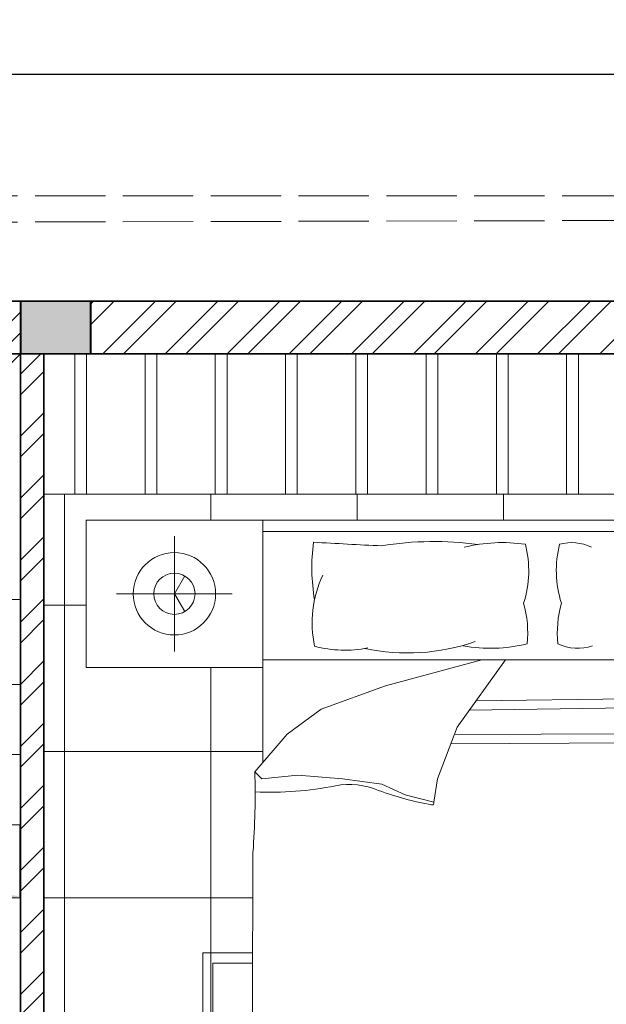
# Model space of a CAD drawing. Units: inches. Extents: x 351 to 1738, y -265 to 286.
# Tile 36 of 38: x 1380 to 1480, y 118 to 286. Entities that reach past the tile are written whole.
import ezdxf

# ---------------------------------------------------------------- set-up
doc = ezdxf.new("R2010")
doc.units = ezdxf.units.IN
doc.header["$MEASUREMENT"] = 0
doc.linetypes.add('ACAD_ISO02W100', pattern=[15, 12, -3])
for name, color, linetype, lineweight in [('A-ANNO-DIMS', 2, 'Continuous', 18), ('A-COLS', 7, 'Continuous', 40), ('A-COLS-PATT', 6, 'Continuous', 13), ('A-FLOR-CASE', 9, 'Continuous', 18), ('A-FLOR-OVHD', 1, 'ACAD_ISO02W100', 18), ('A-FLOR-PATT', 9, 'Continuous', 9), ('A-FLOR-STRS', 7, 'Continuous', 18), ('A-FURN', 18, 'Continuous', 13), ('A-WALL', 7, 'Continuous', 35), ('A-WALL-PATT', 152, 'Continuous', 13)]:
    doc.layers.add(name, color=color, linetype=linetype, lineweight=lineweight)
doc.styles.get("Standard").update_dxf_attribs({"font": 'arial.ttf'})
doc.dimstyles.get("Standard").update_dxf_attribs({"dimtxt": 8, "dimasz": 5, "dimexe": 0.18, "dimexo": 0.0625, "dimgap": 0.09, "dimtad": 1, "dimtoh": 1, "dimzin": 0, "dimdsep": 46, "dimlunit": 4, "dimtxsty": 'Standard', "dimcen": 0, "dimclre": 256, "dimadec": 0, "dimazin": 0, "dimtfac": 1, "dimtofl": 0, "dimtmove": 0, "dimatfit": 3, "dimfxl": 1, "dimtolj": 1, "dimtzin": 0, "dimlwe": -1, "dimarcsym": 0})

# ---------------------------------------------------------------- blocks, each defined once
blk = doc.blocks.new('*D7')
at = {"layer": 'A-ANNO-DIMS', "color": 0, "transparency": 16777216}
for p, q in [((1034.7, 256.03), (1034.7, 276.92)), ((1566.7, 256.03), (1566.7, 276.92))]:
    blk.add_line(p, q, dxfattribs=at)
at = {"layer": 'A-ANNO-DIMS', "color": 0, "lineweight": -2, "transparency": 16777216}
blk.add_line((1039.7, 276.74), (1561.7, 276.74), dxfattribs=at)
at = {"layer": 'A-ANNO-DIMS', "color": 0, "transparency": 16777216}
for points in [[(1039.7, 277.57), (1039.7, 275.91), (1034.7, 276.74)], [(1561.7, 277.57), (1561.7, 275.91), (1566.7, 276.74)]]:
    blk.add_solid(points, dxfattribs=at)
at = {"layer": 'Defpoints', "color": 0, "transparency": 16777216}
for p in [(1566.7, 276.74), (1034.7, 255.96), (1566.7, 255.96)]:
    blk.add_point(p, dxfattribs=at)
at = {"layer": 'A-ANNO-DIMS', "color": 0, "transparency": 16777216, "insert": (1300.7, 280.83), "char_height": 8, "attachment_point": 5}
blk.add_mtext('\\A1;44\'-4"', dxfattribs=at)
blk = doc.blocks.new('*D13')
at = {"layer": 'A-ANNO-DIMS', "color": 0, "transparency": 16777216}
for p, q in [((1338.06, 148.4), (1338.06, 136.03)), ((1380.06, 148.4), (1380.06, 136.03))]:
    blk.add_line(p, q, dxfattribs=at)
at = {"layer": 'A-ANNO-DIMS', "color": 0, "lineweight": -2, "transparency": 16777216}
blk.add_line((1343.06, 136.21), (1375.06, 136.21), dxfattribs=at)
at = {"layer": 'A-ANNO-DIMS', "color": 0, "transparency": 16777216}
for points in [[(1343.06, 137.05), (1343.06, 135.38), (1338.06, 136.21)], [(1375.06, 137.05), (1375.06, 135.38), (1380.06, 136.21)]]:
    blk.add_solid(points, dxfattribs=at)
at = {"layer": 'Defpoints', "color": 0, "transparency": 16777216}
for p in [(1338.06, 148.46), (1380.06, 148.46), (1380.06, 136.21)]:
    blk.add_point(p, dxfattribs=at)
at = {"layer": 'A-ANNO-DIMS', "color": 0, "transparency": 16777216, "insert": (1359.06, 140.39), "char_height": 8, "attachment_point": 5}
blk.add_mtext('\\A1;3\'-6"', dxfattribs=at)
blk = doc.blocks.new('BED-DOUBLE-W-NIGHTSTANDS')
for p, q in [((30.18, 128.33), (30.18, 86.91)), ((120.72, 126.39), (30.18, 126.39)), ((15.09, 105.9), (15.09, 125.61)), ((24.95, 115.76), (5.23, 115.76)), ((30.18, 104.48), (120.72, 104.48)), ((120.32, 98.22), (66.59, 97.46)), ((120.26, 96.67), (65.46, 95.89)), ((120.18, 91.92), (62.88, 91.69)), ((120.19, 90.37), (62.29, 90.13))]:
    blk.add_line(p, q)
for points in [[(30.18, 103.18), (0, 103.18), (0, 128.33), (150.9, 128.33), (150.9, 103.18), (120.72, 103.18), (120.72, 128.33)], [(16.85, 112.71), (15.09, 115.76), (16.85, 118.81)], [(71.64, 104.48), (63.37, 92.97), (60, 84.12), (59.39, 80.15), (54.5, 81.37), (50.53, 83.2), (43.81, 84.12), (36.16, 84.73), (30.05, 84.12), (28.83, 85.34), (34.33, 91.75), (40.14, 96.03), (51.14, 100), (67.6, 104.48)], [(121.56, 54.36), (129.93, 54.36), (129.93, 0), (19.92, 0), (19.92, 54.36), (28.45, 54.36)], [(28.45, 52.61), (21.67, 52.61), (21.67, 1.75), (128.18, 1.75), (128.18, 52.61), (121.53, 52.61)]]:
    blk.add_lwpolyline(points)
for points in [[(38.85, 124.57, 0.074897), (39.03, 114.71, -0.472817)], [(74.74, 114.16, 0.14099), (75.04, 124.22, 0.235245)], [(81.19, 114.16, -0.14099), (80.89, 124.22, -0.235245)], [(28.51, 71.52, 0.001242), (28.44, 42.89, -0.127202), (25.42, 28.62)]]:
    blk.add_lwpolyline(points, format="xyb")
for radius in [7.04, 3.52]:
    blk.add_circle((15.09, 115.76), radius)
for centre, radius, start, end in [((122.02, 1560.65), 1438.48, 266.68521, 267.14978), ((59.52, 69.97), 54.73, 82.2196, 99.497), ((71.08, 97.62), 26.89, 81.5249, 103.96), ((82.96, 117.05), 7.46, 63.3437, 106.1026), ((58.07, 110.76), 19.45, 155.1316, 191.7583), ((56.95, 109.12), 18.49, 354.0129, 15.8293), ((98.98, 109.12), 18.49, 164.1707, 185.9871), ((44.23, 126.34), 20.22, 255.1039, 281.0369), ((54.88, 140.71), 35.07, 258.0397, 289.2615), ((69.08, 133.05), 26.61, 259.8617, 283.6238), ((83.97, 114.44), 8, 245.0183, 288.5407), ((-109.53, 81.59), 138.41, 355.8294, 1.553), ((31.41, 138.78), 56.95, 267.4519, 281.3392), ((45.02, 70.89), 12.28, 66.2616, 101.3392), ((69.87, 137.17), 58.52, 250.1194, 259.3383), ((59.05, 80.02), 0.364, 268.8623, 19.7536)]:
    blk.add_arc(centre, radius, start, end)
blk = doc.blocks.new('WARDROBE-PANELLED')
for p, q in [((5.27, 24), (5.27, 0)), ((7.27, 24), (7.27, 0)), ((17.27, 24), (17.27, 0)), ((19.27, 24), (19.27, 0)), ((29.27, 24), (29.27, 0)), ((31.27, 24), (31.27, 0)), ((41.27, 24), (41.27, 0)), ((43.27, 24), (43.27, 0)), ((53.27, 24), (53.27, 0)), ((55.27, 24), (55.27, 0)), ((65.27, 24), (65.27, 0)), ((67.27, 24), (67.27, 0)), ((77.27, 24), (77.27, 0)), ((79.27, 24), (79.27, 0)), ((89.27, 24), (89.27, 0)), ((91.27, 24), (91.27, 0)), ((0, 0), (173.5, 0))]:
    blk.add_line(p, q)

msp = doc.modelspace()

# ---------------------------------------------------------------- hatches: boundary and pattern name
at = {"layer": 'A-COLS-PATT'}
h = msp.add_hatch(color=256, dxfattribs=at)
h.dxf.hatch_style = 1
h.paths.add_polyline_path([(1112.704, 237.963), (1103.704, 237.963), (1103.704, 228.963), (1112.704, 228.963)])
h.paths.add_polyline_path([(1115.704, 237.963), (1112.704, 237.963), (1112.704, 228.963), (1115.704, 228.963)])
h.paths.add_polyline_path([(1043.704, 255.963), (1034.704, 255.963), (1034.704, 243.963), (1043.704, 243.963)])
h.paths.add_polyline_path([(1043.704, 210.963), (1034.704, 210.963), (1034.704, 198.963), (1043.704, 198.963)])
h.paths.add_polyline_path([(1043.704, -45.037), (1034.704, -45.037), (1034.704, -57.037), (1043.704, -57.037)])
h.paths.add_polyline_path([(1112.704, -45.037), (1103.704, -45.037), (1103.704, -57.037), (1112.704, -57.037)])
h.paths.add_polyline_path([(1112.704, -161.037), (1103.704, -161.037), (1103.704, -164.037), (1103.704, -173.037), (1112.704, -173.037)])
h.paths.add_polyline_path([(1043.704, -161.037), (1034.704, -161.037), (1034.704, -173.037), (1043.704, -173.037)])
h.paths.add_polyline_path([(1248.549, -164.037), (1236.549, -164.037), (1236.549, -173.037), (1248.549, -173.037)])
h.paths.add_polyline_path([(1248.549, -50), (1236.549, -50), (1236.549, -59), (1248.549, -59)])
h.paths.add_polyline_path([(1248.704, 73.463), (1244.704, 73.463), (1244.704, 64.463), (1248.704, 64.463)])
h.paths.add_polyline_path([(1244.704, 73.463), (1236.704, 73.463), (1236.704, 64.463), (1244.704, 64.463)])
h.paths.add_polyline_path([(1248.704, 237.963), (1236.704, 237.963), (1236.704, 228.963), (1248.704, 228.963)])
h.paths.add_polyline_path([(1392.204, 237.963), (1380.204, 237.963), (1380.204, 228.963), (1392.204, 228.963)])
h.paths.add_polyline_path([(1536.064, 237.963), (1524.064, 237.963), (1524.064, 228.963), (1536.064, 228.963)])
h.paths.add_polyline_path([(1536.064, 73.463), (1524.064, 73.463), (1524.064, 64.463), (1536.064, 64.463)])
h.paths.add_polyline_path([(1384.204, 73.463), (1380.204, 73.463), (1380.204, 64.463), (1384.204, 64.463)])
h.paths.add_polyline_path([(1392.064, 73.463), (1384.204, 73.463), (1384.204, 64.463), (1392.064, 64.463)])
h.paths.add_polyline_path([(1536.064, -53.037), (1524.064, -53.037), (1524.064, -57.037), (1536.064, -57.037)])
h.paths.add_polyline_path([(1536.064, -48.037), (1524.064, -48.037), (1524.064, -53.037), (1536.064, -53.037)])
h.paths.add_polyline_path([(1392.064, -48.037), (1380.064, -48.037), (1380.064, -56.5), (1380.065, -57.037), (1392.064, -57.037)])
h.paths.add_polyline_path([(1536.064, -164.037), (1524.064, -164.037), (1524.064, -173.037), (1536.064, -173.037)])
at = {"layer": 'A-FLOR-PATT', "transparency": 33554559}
h = msp.add_hatch(dxfattribs=at)
h.set_pattern_fill('ANSI37', color=256, scale=200, angle=135)
h.set_pattern_definition([(180, (1112.704, -164.037), (-2e-15, -25), []), (270, (1112.704, -164.037), (25, -5e-15), [])])
h.paths.add_polyline_path([(1380.064, 73.463), (1380.132, 148.463), (1338.064, 148.463), (1290.704, 148.463), (1290.704, 88.463), (1248.704, 88.463), (1248.704, -2.009), (1244.704, -2.009), (1244.704, 142.457), (1160.704, 142.457), (1160.704, 158.963), (1160.704, 170.137), (1160.704, 206.137), (1160.704, 228.963), (1112.704, 228.963), (1112.704, 209.963), (1112.704, 168.963), (1124.704, 168.963), (1124.704, 162.963), (1112.704, 162.963), (1112.704, 64.463), (1112.704, 60.463), (1112.704, 0.463), (1112.704, -48.026), (1146.804, -47.981), (1146.804, -35.691), (1207.804, -35.691), (1207.804, -47.902), (1236.542, -47.864), (1236.544, -50.009), (1248.5, -50.009), (1248.506, -102.915), (1248.512, -150.915), (1248.514, -164.037), (1248.549, -164.037), (1273.017, -164.037), (1273.017, -128.799), (1355.24, -128.799), (1355.24, -164.037), (1384.204, -164.037), (1384.204, -57.037), (1380.064, -57.037), (1380.064, -48.037), (1392.064, -48.037), (1392.064, -53.037), (1406.549, -53.037), (1406.549, -57.037), (1401.204, -57.037), (1401.204, -147.037), (1468.204, -147.037), (1468.204, -138.5), (1472.204, -138.5), (1472.204, -102.5), (1468.204, -102.5), (1468.204, -57.037), (1442.549, -57.037), (1442.549, -53.037), (1463.049, -53.037), (1463.049, -40.747), (1524.049, -40.747), (1524.049, -48.037), (1536.064, -48.037), (1536.064, -53.037), (1557.704, -53.037), (1557.704, 204.963), (1384.204, 204.963), (1384.204, 73.463), (1392.064, 73.463), (1392.064, 64.463), (1384.204, 64.463), (1384.204, -3.5), (1380.204, -3.537), (1380.204, 64.463), (1380.064, 64.463)])
h.paths.add_polyline_path([(1510.714, 86.458, -0.1039845), (1511.661, 85.595, 0.4704384), (1510.158, 87.614, 0.0961001)], flags=16)
h.paths.add_polyline_path([(1510.443, 100.266, 0.009798), (1504.693, 100.48, 0.0287898), (1504.6, 99.767, -0.1653311), (1505.519, 96.135, -0.1436014)], flags=16)
h.paths.add_polyline_path([(1487.201, 85.595, -0.1039845), (1488.148, 86.458, 0.0961001), (1488.704, 87.614, 0.4704384)], flags=0)
h.paths.add_polyline_path([(1495.052, 100.43), (1494.178, 100.43, -0.0264629), (1494.262, 99.774, -0.1442193)], flags=16)
h.paths.add_polyline_path([(1444.485, 86.458, -0.1039845), (1445.433, 85.595, 0.4704384), (1443.93, 87.614, 0.0961001)], flags=16)
h.paths.add_polyline_path([(1420.972, 85.595, -0.1039845), (1421.92, 86.458, 0.0961001), (1422.475, 87.614, 0.4704384)], flags=16)
h.paths.add_polyline_path([(1428.632, 100.335, 0.0010541), (1427.971, 100.309, -0.0215241), (1428.033, 99.774, -0.1143008)], flags=16)
h.paths.add_polyline_path([(1419.906, 143.708, 0.0249793), (1420.222, 157.526), (1421.573, 159.101), (1421.573, 175.369), (1391.393, 175.369), (1391.393, 200.519), (1542.294, 200.519), (1542.294, 175.369), (1512.028, 175.369, 0.0198653), (1511.521, 153.838, 0.0251335), (1512.758, 118.323, 0.0205529), (1512.942, 115.253), (1419.834, 115.253, -0.0004142), (1419.843, 124.798), (1413.059, 124.798), (1413.059, 84.437, -0.0618528), (1415.831, 80.45, -0.0930773), (1420.972, 85.595, -0.2675367), (1422.371, 84.732, 0.0851103), (1424.052, 84.616, -0.8853927), (1424.033, 84.851, -1.1258145), (1424.073, 84.366, -0.0879871), (1422.371, 84.732, -0.2675367), (1422.326, 83.089, -0.3705421), (1420.972, 85.595, 0.0930773), (1415.831, 80.45, -0.0874142), (1417.914, 73.937), (1418.941, 73.937, 0.0272504), (1418.913, 76.906, -0.1157032), (1421.051, 73.937), (1445.354, 73.937, -0.1157032), (1447.492, 76.906, 0.0272504), (1447.464, 73.937), (1448.491, 73.937, -0.0874142), (1450.574, 80.45, 0.0930773), (1445.433, 85.595, -0.3705421), (1444.079, 83.089, -0.2675367), (1444.034, 84.732, -0.0879871), (1442.332, 84.366, -1.1258145), (1442.372, 84.851, -2.0327363), (1442.364, 84.368, 0.0863779), (1444.034, 84.732, -0.2675367), (1445.433, 85.595, -0.0930773), (1450.574, 80.45, -0.2577317), (1466.483, 90.927, -0.4786702), (1468.832, 91.907, -0.4786702), (1471.18, 90.927, -0.26264), (1483.053, 81.78, -0.0718662), (1487.201, 85.595, -0.2675367), (1488.6, 84.732, 0.0851103), (1490.28, 84.616, -0.8853927), (1490.262, 84.851, -1.1258145), (1490.301, 84.366, -0.0879871), (1488.6, 84.732, -0.2675367), (1488.554, 83.089, -0.3705421), (1487.201, 85.595, 0.0718662), (1483.053, 81.78, -0.1320648), (1484.143, 73.937), (1485.169, 73.937, 0.0272504), (1485.142, 76.906, -0.1157032), (1487.28, 73.937), (1511.582, 73.937, -0.1157032), (1513.72, 76.906, 0.0272504), (1513.693, 73.937), (1514.719, 73.937, -0.0874142), (1516.802, 80.45, 0.0930773), (1511.661, 85.595, -0.3705421), (1510.308, 83.089, -0.2675367), (1510.262, 84.732, -0.0879871), (1508.561, 84.366, -1.1258145), (1508.601, 84.851, -2.0327363), (1508.592, 84.368, 0.0863779), (1510.262, 84.732, -0.2675367), (1511.661, 85.595, -0.0930773), (1516.802, 80.45, -0.0618528), (1519.575, 84.437), (1519.575, 73.937), (1413.059, 73.937), (1413.059, 124.798), (1419.843, 124.798, -0.0008205)], flags=16)
h.paths.add_polyline_path([(1220.149, 54.133, -0.1039845), (1220.869, 53.476, 0.4704384), (1219.727, 55.011, 0.0961001)], flags=16)
h.paths.add_polyline_path([(1219.944, 64.626, 0.009798), (1215.574, 64.789, 0.0287898), (1215.503, 64.247, -0.1653311), (1216.201, 61.487, -0.1436014)], flags=16)
h.paths.add_polyline_path([(1209.779, 64.449, 0.0974459), (1209.339, 64.751), (1208.247, 64.751, 0.1273905), (1207.7, 64.326, 0.1715858), (1206.95, 61.475, -0.1588542), (1207.636, 59.45, 0.0158984), (1207.795, 59.218, 0.0615457), (1208.598, 59.616, 0.1754158), (1208.638, 60.099, -0.2847793), (1209.348, 62.472, 0.3262165)], flags=16)
h.paths.add_polyline_path([(1169.818, 54.133, -0.1039845), (1170.538, 53.476, 0.4704384), (1169.396, 55.011, 0.0961001)], flags=16)
h.paths.add_polyline_path([(1159.017, 62.472, 0.2847642), (1158.307, 60.099, -0.1754332), (1158.267, 59.616, 0.3929302), (1159.448, 64.449, -0.3262298)], flags=16)
h.paths.add_polyline_path([(1156.342, 58.239, -0.1783213), (1154.011, 55.31, -0.1747359), (1154.722, 55.233, -0.2008015), (1156.27, 56.086, 0.1269899), (1157.283, 58.991, -0.0912053)], flags=16)
h.paths.add_polyline_path([(1156.624, 61.413, 0.1572752), (1157.316, 64.247, 0.1696217)], flags=16)
h.paths.add_polyline_path([(1152.67, 54.133, -0.0961001), (1151.95, 53.476, 0.0640762), (1154.465, 54.384, 0.1990158)], flags=16)
h.paths.add_polyline_path([(1202.281, 53.476, -0.1039845), (1203, 54.133, 0.0961001), (1203.423, 55.011, 0.4704384)], flags=0)
h.paths.add_polyline_path([(1151.139, 97.64, 0.0249793), (1151.379, 108.141), (1152.406, 109.338), (1152.406, 121.701), (1129.47, 121.701), (1129.47, 140.814), (1244.149, 140.814), (1244.149, 121.701), (1221.148, 121.701, 0.0198653), (1220.763, 105.338, 0.0251335), (1221.703, 78.349, 0.0205529), (1221.843, 76.016), (1151.078, 76.016, -0.1287433), (1148.786, 65.037, 0.5393525), (1150.327, 64.171, -0.027594), (1163.481, 64.751, 0.0976954), (1163.04, 64.449, 0.3262165), (1163.471, 62.472, -0.2847765), (1164.181, 60.099, -0.1947567), (1165.846, 61.443, -0.1554021), (1165.172, 64.247, -0.1660224), (1165.869, 61.475, -0.1770142), (1167.852, 62.77, -0.4482027), (1169.974, 60.807, -0.3934987), (1167.679, 57.86, -0.8955483), (1168.438, 54.524, -0.3557668), (1166.218, 56.086, -0.066024), (1165.505, 57.539), (1165.251, 56.243, -0.3717324), (1164.02, 59.758, -0.3736141), (1163.04, 64.449, -0.0976954), (1163.481, 64.751, 0.0213538), (1153.294, 64.429, -0.1341826), (1156.695, 61.368, 0.1868727), (1154.636, 62.77, 0.4482027), (1152.514, 60.807, 0.4037263), (1154.905, 57.846, 0.7112192), (1153.334, 55, 0.5315397), (1151.95, 53.476, -0.2675367), (1153.013, 52.821, 0.0851103), (1154.29, 52.732, -0.8853927), (1154.276, 52.911, -1.1258145), (1154.306, 52.543, -0.0879871), (1153.013, 52.821, -0.2675367), (1152.978, 51.572, -0.3705421), (1151.95, 53.476, 0.0930773), (1148.043, 49.566, -0.0874142), (1149.626, 44.617), (1150.406, 44.617, 0.0272504), (1150.385, 46.873, -0.1157032), (1152.01, 44.617), (1170.478, 44.617, -0.1157032), (1172.103, 46.873, 0.0272504), (1172.082, 44.617), (1172.862, 44.617, -0.0874142), (1174.445, 49.566, 0.0930773), (1170.538, 53.476, -0.3705421), (1169.51, 51.572, -0.2675367), (1169.475, 52.821, -0.0879871), (1168.182, 52.543, -1.1258145), (1168.212, 52.911, -2.0327363), (1168.206, 52.544, 0.0863779), (1169.475, 52.821, -0.2675367), (1170.538, 53.476, -0.0930773), (1174.445, 49.566, -0.2577317), (1186.536, 57.528, -0.4786702), (1188.321, 58.273, -0.4786702), (1190.106, 57.528, -0.26264), (1199.128, 50.577, -0.0718662), (1202.281, 53.476, -0.2675367), (1203.344, 52.821, 0.0851103), (1204.621, 52.732, -0.8853927), (1204.607, 52.911, -1.1258145), (1204.637, 52.543, -0.0879871), (1203.344, 52.821, -0.2675367), (1203.309, 51.572, -0.3705421), (1202.281, 53.476, 0.0718662), (1199.128, 50.577, -0.1320648), (1199.957, 44.617), (1200.737, 44.617, 0.0272504), (1200.716, 46.873, -0.1157032), (1202.341, 44.617), (1220.809, 44.617, -0.1157032), (1222.434, 46.873, 0.0272504), (1222.413, 44.617), (1223.193, 44.617, -0.0874142), (1224.776, 49.566, 0.0930773), (1220.869, 53.476, -0.3705421), (1219.841, 51.572, -0.2675367), (1219.806, 52.821, -0.0879871), (1218.513, 52.543, -1.1258145), (1218.543, 52.911, -2.0327363), (1218.537, 52.544, 0.0863779), (1219.806, 52.821, -0.2675367), (1220.869, 53.476, -0.0930773), (1224.776, 49.566, -0.0618528), (1226.883, 52.597), (1226.883, 44.617), (1145.936, 44.617), (1145.936, 83.269), (1151.091, 83.269, -0.0008205)], flags=16)
h.paths.add_polyline_path([(1218.01, 57.86, -0.8955483), (1218.769, 54.524, -0.3557668), (1216.549, 56.086, -0.066024), (1215.836, 57.539), (1215.582, 56.243, -0.3717324), (1214.351, 59.758, -0.3736141), (1213.371, 64.449, 0.3262165), (1213.802, 62.472, -0.2847765), (1214.512, 60.099, -0.1947567), (1216.177, 61.443, -0.1799907), (1218.183, 62.77, -0.4482027), (1220.305, 60.807, -0.3934987)], flags=16)
h.paths.add_polyline_path([(1424.735, 91.363, -0.3934987), (1421.715, 95.241, -0.4482027), (1424.507, 97.824, -0.1799907), (1427.147, 96.077, -0.1947567), (1429.338, 94.309, -0.2847765), (1430.272, 97.432, 0.3262165), (1430.839, 100.034, -0.3736141), (1429.55, 93.861, -0.3717324), (1427.929, 89.235), (1427.596, 90.941, -0.066024), (1426.657, 89.029, -0.3557668), (1423.736, 86.973, -0.8955483)], flags=16)
h.paths.add_polyline_path([(1238.033, 131.257, -1), (1227.329, 131.257, -1)], flags=0)
h.paths.add_polyline_path([(1235.357, 131.257, -1), (1230.005, 131.257, -1)], flags=0)
h.paths.add_polyline_path([(1214.039, 54.243, 0.1543819), (1214.38, 53.992, 0.3589549), (1213.613, 54.016, 0.6039484), (1214.379, 53.657, 0.3713191), (1213.968, 52.872, 0.1879935), (1214.312, 52.809, -0.592455), (1213.953, 52.967, -0.2942791), (1214.083, 53.691, -1.3001871), (1213.881, 54.134, -0.2837621), (1214.469, 53.896, 1.1509396)], flags=16)
h.paths.add_polyline_path([(1212.091, 56.286, -0.4084338), (1211.337, 56.445, -0.0362594), (1211.098, 56.848, -0.2360976), (1211.59, 56.63, 0.0353445), (1211.835, 56.543, -0.4752408), (1212.091, 56.286, -0.4752408), (1212.438, 56.182, 0.0353445), (1212.631, 56.007, -0.2360976), (1213.056, 55.676, -0.0362594), (1212.588, 55.697, -0.4084338)], flags=16)
h.paths.add_polyline_path([(1211.469, 50.297, 0.296043), (1210.47, 50.527, 0.310883), (1211.931, 50.148, 0.0212546)], flags=16)
h.paths.add_polyline_path([(1213.739, 51.818, -0.0362594), (1213.271, 51.838, -0.4084337), (1212.774, 52.427, -0.0947856), (1212.293, 50.703, 1.1504738), (1212.911, 50.232, 0.1662877), (1213.265, 50.68, -0.0252543), (1212.603, 50.13, 1.0879317), (1212.471, 49.407, 0.1662877), (1213.02, 49.251, -0.016128), (1212.567, 49.563, -0.286859), (1212.217, 49.638, 0.0221563), (1212.046, 50.055, -0.6461302), (1212.185, 50.498, 0.0884116), (1212.732, 52.077, -1.1860374), (1213.121, 52.323, 0.0353445), (1213.314, 52.148, -0.2360976)], flags=16)
h.paths.add_polyline_path([(1212.094, 50.342, -0.0485241), (1211.54, 49.605, -1.1038339), (1211.397, 48.738, -0.7855147), (1211.683, 48.254, -0.3920429), (1210.948, 48.525, -0.3928194), (1210.561, 47.995, -0.592455), (1210.201, 48.153, -0.2942791), (1210.331, 48.877, -0.7041716), (1210.316, 49.592, -0.6793441), (1210.729, 50.112, 0.5636764)], flags=16)
h.paths.add_polyline_path([(1211.274, 49.829, -0.1398258), (1210.745, 49.859, -0.2178785), (1210.948, 49.509, -0.4985724)], flags=0)
h.paths.add_polyline_path([(1433.426, 81.49, -0.181571), (1434.245, 81.788, -0.0080665), (1433.726, 82.205, 0.0455784), (1432.755, 81.242, 0.1790113)], flags=16)
h.paths.add_polyline_path([(1434.146, 81.009, -0.1324418), (1433.645, 80.771, 0.2590893), (1433.234, 80.471, -0.1802109), (1433.392, 80.805, -0.1699398), (1432.758, 81.109, 0.0326525), (1433.273, 80.474, -0.4933627), (1434.046, 80.146, -0.3904966)], flags=16)
h.paths.add_polyline_path([(1434.83, 80.047, -0.9475376), (1435.294, 79.576, -0.2991282), (1434.625, 79.404, -0.2704392), (1435.01, 78.591, -0.592455), (1434.537, 78.382, -0.3928194), (1434.027, 79.08, -0.3920429), (1433.06, 78.723, -0.3520423), (1433.003, 79.197, -0.1972159), (1433.75, 79.734, -0.7136405), (1434.447, 79.939, -0.2147903), (1434.819, 80.475, 0.4088333), (1435.075, 80.803, -0.2261519)], flags=16)
h.paths.add_polyline_path([(1432.67, 81.217, -0.4542182), (1431.897, 79.923, -0.4144105), (1431.301, 80.035, 0.0161291), (1431.897, 80.445, 0.2795702), (1432.073, 80.871, -0.2895037), (1431.103, 81.321, -0.4144105), (1430.978, 81.915, 0.0161296), (1431.586, 81.521, 0.341293), (1432.125, 81.583, -0.8131856)], flags=16)
h.paths.add_polyline_path([(1429.893, 86.381, -0.9475376), (1430.358, 85.91, -0.1731062), (1429.984, 85.712, -0.0388172), (1431.625, 84.214, -0.0879005), (1432.097, 88.549, -0.0497684), (1431.254, 88.49, -0.2360976), (1431.814, 88.925, 0.0353445), (1432.067, 89.155, -0.4752408), (1432.524, 89.291, -0.4752408), (1432.86, 89.63, 0.0353445), (1433.182, 89.744, -0.2360976), (1433.83, 90.032, -0.0362594), (1433.516, 89.502, -0.4084338), (1432.524, 89.291, -0.3124239), (1432.106, 88.58, 0.0885594), (1431.625, 84.214, -0.4084337), (1430.971, 83.439, -0.0362594), (1430.355, 83.412, -0.2360976), (1430.914, 83.847, 0.0353445), (1431.168, 84.078, -0.4752408), (1431.625, 84.214, 0.0388172), (1429.984, 85.712, -0.3217316), (1429.333, 86.048, -0.32743), (1429.883, 86.809, 0.4088333), (1430.138, 87.138, -0.2261519)], flags=16)
h.paths.add_polyline_path([(1211.206, 58.616, -0.9997836), (1211.336, 59.323, -0.6149935)], flags=16)
h.paths.add_polyline_path([(1210.288, 49.429, 0.1543819), (1210.629, 49.178, 0.3589549), (1209.861, 49.202, 0.6039484), (1210.627, 48.843, -0.5348247), (1210.806, 49.295, 0.7483464)], flags=16)
h.paths.add_polyline_path([(1209.589, 51.828, -0.0087906), (1209.775, 51.753, 0.1122315), (1209.466, 52.019, 1.4188509), (1209.014, 51.708, -0.4587257), (1208.651, 51.073, -0.592455), (1208.291, 51.232, -0.2942791), (1208.421, 51.955, -1.3001871), (1208.219, 52.398, -0.2260052), (1208.719, 52.257, -0.4755189), (1209.158, 52.369, -1.4554994), (1209.603, 52.664, 0.4213049), (1209.191, 52.262, -0.5912116), (1208.979, 51.796, 0.4973986), (1209.773, 51.333, 0.6493116)], flags=16)
h.paths.add_polyline_path([(1208.029, 52.041, 0.5446671), (1208.832, 52.045, 0.220132)], flags=0)
h.paths.add_polyline_path([(1210.438, 51.425, -0.2041997), (1210.277, 52.018, 0.2708262), (1209.915, 52.897, 0.3241145)], flags=0)
h.paths.add_polyline_path([(1209.668, 52.407, -0.60139), (1208.99, 52.221, -0.3949159), (1208.248, 52.83, -0.8367916), (1208.651, 53.017, -0.3384876), (1209.039, 52.571, 0.1941379), (1209.191, 52.262, 0.4139945), (1209.712, 52.475, 0.5177103), (1210.503, 51.416, 0.401922), (1209.493, 50.93, 0.2063956), (1209.516, 50.165, -0.3194629), (1210.417, 51.418, -0.466635)], flags=16)
h.paths.add_polyline_path([(1206.601, 56.086, -0.3557668), (1204.381, 54.524, -0.9211983), (1205.236, 57.846, 0.2065693), (1207.614, 58.991, -0.1269899)], flags=16)
h.paths.add_polyline_path([(1435.487, 82.816, 0.5277653), (1436.615, 83.361, 0.5085402), (1437.05, 82.433, 0.592455), (1437.524, 82.641, 0.3312448), (1436.963, 83.548, 0.3878632), (1437.808, 83.626, 0.5929544), (1437.618, 84.176, 0.2260158), (1436.961, 83.99, 0.3182053), (1437.588, 84.854, 0.6893744), (1437.05, 84.991, 0.3357648), (1436.539, 84.41, -0.1569934), (1436.404, 84.065, -0.4346112), (1436.961, 83.99, -0.2147903), (1437.333, 84.526, 0.4088333), (1437.588, 84.854, -0.2261519), (1437.343, 84.097, -0.9475376), (1437.808, 83.626, -0.2991282), (1437.139, 83.455, -0.2704392), (1437.524, 82.641, -0.592455), (1437.05, 82.433, -0.3928194), (1436.541, 83.13, -0.4396601), (1435.475, 82.794, -0.174614), (1435.942, 82.244, -0.2063956), (1435.912, 81.237, -0.2708262), (1435.125, 82.208, 0.2079765), (1434.686, 82.904, -0.1964955)], flags=16)
h.paths.add_polyline_path([(1435.386, 84.832, 0.270811), (1434.91, 83.676, -0.2042174), (1434.699, 82.895, 0.3241145)], flags=0)
h.paths.add_polyline_path([(1435.68, 84.18, -0.2176564), (1435.554, 83.304, -0.1767045), (1436.236, 83.778, -0.3730364)], flags=0)
h.paths.add_polyline_path([(1435.566, 100.034, 0.3262165), (1436.133, 97.432, -0.2847765), (1437.067, 94.309, -0.1947567), (1439.258, 96.077, -0.1554021), (1438.371, 99.767, -0.1660224), (1439.289, 96.12, -0.1770142), (1441.897, 97.824, -0.4482027), (1444.69, 95.241, -0.3934987), (1441.67, 91.363, -0.8955483), (1442.669, 86.973, -0.3557668), (1439.748, 89.029, -0.066024), (1438.809, 90.941), (1438.476, 89.235, -0.3717324), (1436.855, 93.861, -0.3736141)], flags=16)
h.paths.add_polyline_path([(1191.252, 49.507, -0.2740221), (1190.658, 48.409, 0.2675367), (1191.311, 47.344, 0.3705421)], flags=0)
h.paths.add_polyline_path([(1190.301, 49.717, 0.1990158), (1188.619, 49.04, 0.0640762), (1191.252, 49.507, -0.0961001)], flags=0)
h.paths.add_polyline_path([(1189.518, 47.857, 1.1258145), (1189.676, 47.523, 2.0446052)], flags=0)
h.paths.add_polyline_path([(1464.974, 80.372, 0.2740221), (1465.756, 78.927, -0.0830131)], flags=0)
h.paths.add_polyline_path([(1464.974, 80.372, 0.3705421), (1464.897, 77.525, 0.5763244)], flags=0)
h.paths.add_polyline_path([(1464.974, 80.372, -0.4704384), (1467.284, 81.372, -0.0961001), (1466.226, 80.648, -0.1990158), (1468.439, 79.757, -0.0640762)], flags=0)
h.paths.add_polyline_path([(1189.511, 56.43, -0.2594668), (1188.321, 56.391, -0.2594668), (1187.13, 56.43, 0.0851103), (1188.193, 55.716, -0.8853927), (1188.27, 55.878, -1.1960133), (1188.355, 55.442, 0.1014587)], flags=0)
h.paths.add_polyline_path([(1188.321, 57.596, 0.0780722), (1187.678, 57.24, 0.0155503), (1188.321, 57.136, 0.0155503), (1188.964, 57.24, 0.0780722)], flags=0)
h.paths.add_polyline_path([(1190.164, 55.365, -0.5763244), (1190.106, 57.528, -0.1982945), (1188.321, 58.319, -0.1982945), (1186.536, 57.528, -0.5763244), (1186.477, 55.365, -0.3705421), (1186.536, 57.528, 0.1982945), (1188.321, 58.319, 0.1982945), (1190.106, 57.528, -0.3705421)], flags=0)
h.paths.add_polyline_path([(1188.372, 55.878, 1.1258145), (1188.529, 55.544, 2.0446052)], flags=0)
h.paths.add_polyline_path([(1186.341, 49.717, -0.0961001), (1185.389, 49.507, 0.0640762), (1188.022, 49.04, 0.1990158)], flags=0)
h.paths.add_polyline_path([(1185.389, 49.507, -0.2675367), (1185.984, 48.409, 0.0851103), (1187.046, 47.695, -0.8853927), (1187.123, 47.857, -1.1258145), (1186.966, 47.523, -0.0879871), (1185.984, 48.409, -0.2675367), (1185.331, 47.344, -0.3705421)], flags=0)
h.paths.add_polyline_path([(1399.441, 187.944, -1), (1413.525, 187.944, -1)], flags=0)
h.paths.add_polyline_path([(1402.962, 187.944, -1), (1410.004, 187.944, -1)], flags=0)
h.paths.add_polyline_path([(1357.663, -72.245), (1377.272, -72.245), (1377.272, -91.854), (1357.663, -91.854)], flags=16)
h.paths.add_polyline_path([(1467.256, 78.201, -1.1258145), (1467.049, 77.761, -2.0446052)], flags=0)
h.paths.add_polyline_path([(1468.822, 88.714, 0.9411249), (1469.106, 88.316, 1.1371523), (1468.765, 88.755, 0.890986), (1468.99, 88.245, 0.0948283), (1470.398, 89.481, -0.2675367), (1471.18, 90.927, -0.0281232), (1469.678, 90.547, -0.0287737), (1469.948, 90.311, -0.0203267), (1468.832, 90.41, -0.0203267), (1467.716, 90.311, -0.0287737), (1467.986, 90.547, -0.0281232), (1466.483, 90.927, -0.2675367), (1467.265, 89.481, 0.0851103), (1468.663, 88.542, -1.2023159)], flags=0)
h.paths.add_polyline_path([(1178.25, 124.523, -0.1199286), (1165.65, 124.145, -0.1073492), (1159.133, 124.446, -0.1028906), (1159.132, 130.465, -0.0748968), (1158.993, 137.956, 0.002027), (1167.844, 137.479, -0.07553), (1180.337, 137.666, -0.0758613), (1186.502, 137.688, -0.1409896), (1186.272, 130.046, -0.0954805), (1186.729, 124.748, -0.10603)], flags=0)
h.paths.add_polyline_path([(1469.225, 79.757, -0.1990158), (1471.437, 80.648, -0.0961001), (1470.379, 81.372, -0.4704384), (1472.689, 80.372, -0.3705421), (1472.766, 77.525, -0.2675367), (1471.907, 78.927, -0.0879863), (1470.615, 77.761, -1.1258491), (1470.408, 78.201, -2.0327363), (1470.642, 77.778, 0.0863779), (1471.907, 78.927, -0.2675367), (1472.689, 80.372, -0.0640762)], flags=0)
h.paths.add_polyline_path([(1430.423, 186.902, -0.0748968), (1430.24, 196.758, 0.002027), (1441.887, 196.131, -0.07553), (1458.326, 196.377, -0.0758613), (1466.438, 196.406, -0.1409896), (1466.136, 186.35, -0.0954805), (1466.737, 179.378, -0.10603), (1455.58, 179.082, -0.1199286), (1439, 178.585, -0.1073492), (1430.425, 178.981, -0.1028906)], flags=0)
h.paths.add_polyline_path([(1162.258, 49.939, 0.3357645), (1161.87, 49.497, -0.1569936), (1161.767, 49.235, -0.4346112), (1162.19, 49.178, -0.2147903), (1162.473, 49.585, 1.5291948)], flags=16)
h.paths.add_polyline_path([(1161.683, 49.021, 0.5815181), (1161.268, 49.583, 0.5927609)], flags=16)
h.paths.add_polyline_path([(1162.602, 48.058, 0.3713191), (1162.192, 48.843, 0.4345332), (1162.88, 48.962, 0.1850806), (1162.197, 48.926, 1.1218369)], flags=16)
h.paths.add_polyline_path([(1161.443, 48.941, -1.3071038), (1161.495, 48.571, -0.2177521), (1161.136, 48.254, 0.6973029), (1161.871, 49.048, 0.1215141)], flags=16)
h.paths.add_polyline_path([(1162.531, 49.429, -0.2070837), (1162.05, 49.146, -0.9920299)], flags=16)
h.paths.add_polyline_path([(1161.304, 49.578, -0.7196675), (1161.513, 50.079, -0.1304275), (1160.836, 50.168, 0.0395926)], flags=0)
h.paths.add_polyline_path([(1162.036, 50.584, -0.0080665), (1161.642, 50.9, 0.0293675), (1161.35, 50.297, -0.2057884)], flags=16)
h.paths.add_polyline_path([(1162.882, 51.392, -0.1247327), (1162.763, 51.828, -0.1011907), (1162.399, 51.438, -0.153425)], flags=0)
h.paths.add_polyline_path([(1164.235, 51.85, -0.3091075), (1164.513, 51.136, -0.6271245), (1163.781, 51.603, -0.6859091), (1162.777, 51.219, -0.2332851), (1163.303, 50.165, -0.2708262), (1162.705, 50.903, 0.2041997), (1162.381, 51.425, 0.204182), (1162.542, 52.018, -0.2708414), (1162.903, 52.897, -0.1272607), (1163.219, 52.529, -1.1686811), (1163.781, 52.587, -0.3291117), (1164.168, 53.017, -0.8367917), (1164.571, 52.83, -0.1933406), (1164.391, 52.338, -0.9475376), (1164.744, 51.981, -0.2991282)], flags=16)
h.paths.add_polyline_path([(1163.598, 51.937, -1.2629561), (1163.236, 51.831, 0.0125754), (1162.971, 51.721, 0.2306566), (1163.151, 52.407, -0.1648982), (1163.178, 52.661, -0.4493201), (1163.628, 52.262, -0.721477), (1164.154, 52.088, -0.8499982)], flags=0)
h.paths.add_polyline_path([(1161.613, 58.616, -0.9804131), (1161.525, 59.049, -2.9089348)], flags=16)
h.paths.add_polyline_path([(1160.252, 49.166, -0.4144105), (1159.799, 49.251, 0.0161291), (1160.252, 49.563, 0.2795702), (1160.386, 49.887, -0.2895037), (1159.649, 50.229, -0.4144105), (1159.554, 50.68, 0.0161296), (1160.015, 50.381, 0.6178854), (1160.526, 50.703, -0.0947856), (1160.045, 52.427, -0.1404436), (1159.682, 52.042, -0.0578559), (1159.3, 51.872, 0.5448433), (1160.046, 52.419, -0.0881216), (1160.404, 55.721, -0.0497684), (1159.763, 55.676, -0.2360976), (1160.188, 56.007, 0.0353445), (1160.381, 56.182, -0.4752408), (1160.728, 56.286, -0.4752408), (1160.984, 56.543, 0.0353445), (1161.229, 56.63, -0.2360976), (1161.721, 56.848, -0.0362594), (1161.482, 56.445, -0.4084338), (1160.728, 56.286, -0.3124239), (1160.411, 55.745, 0.0885594), (1160.045, 52.427, 0.1070813), (1160.634, 50.498, -0.4947977), (1160.839, 50.149, -0.4542182)], flags=16)
h.paths.add_polyline_path([(1160.666, 49.808, -2.0765276), (1160.828, 50.172, 0.0195861)], flags=0)
h.paths.add_polyline_path([(1158.439, 53.992, 0.1543819), (1158.78, 54.243, 0.7483463), (1158.262, 54.109, -0.3382251), (1158.492, 53.839, -0.1708158), (1159.124, 53.779, 0.4957286), (1158.938, 54.134, 0.2260157)], flags=16)
h.paths.add_polyline_path([(1160.045, 52.427, 0.0388172), (1158.798, 53.565, -0.1198178), (1158.574, 53.586, -0.3091075), (1158.851, 52.872, -0.1879935), (1158.506, 52.809, 0.592455), (1158.866, 52.967, 0.3312448), (1158.44, 53.657, 0.2012451), (1158.798, 53.565, -0.034023), (1159.901, 52.578, -0.0442527), (1159.698, 52.323, -0.4752408)], flags=16)
h.paths.add_polyline_path([(1336.926, -95.392), (1336.926, -117.945), (1291.82, -117.945), (1291.82, -95.392)], flags=16)
h.paths.add_polyline_path([(1357.535, -97.244), (1357.726, -96.697, 0.0348443)], flags=16)
h.paths.add_polyline_path([(1376.693, -96.478), (1377.301, -96.5, 0.0314968), (1375.907, -96.424), (1357.726, -96.424)], flags=16)
h.paths.add_polyline_path([(1379.403, -119.667, 0.0267056), (1380.043, -119.439, -0.0152991)], flags=16)
h.paths.add_polyline_path([(1357.726, -120.202), (1357.821, -120.202), (1357.821, -120.201)], flags=16)
h.paths.add_polyline_path([(1354.171, -104.592), (1354.469, -98.672, 0.0111377)], flags=16)
h.paths.add_polyline_path([(1355.058, -119.136), (1354.578, -118.539, 0.1431635)], flags=16)
h.paths.add_polyline_path([(1378.851, -96.821), (1378.85, -96.82), (1378.85, -96.82, -0.0496798), (1380.055, -97.191), (1378.85, -96.82, 0.1500541), (1375.135, -97.188), (1375.136, -119.44, -0.0099698), (1374.747, -116.649), (1357.726, -116.649, 0.1693849), (1357.535, -119.382), (1357.535, -119.382), (1357.535, -119.382, 0.0348176), (1357.726, -119.928), (1357.726, -119.928), (1357.726, -119.929, -0.0348772), (1357.535, -119.382), (1355.507, -119.382), (1355.317, -119.278), (1357.535, -119.382, -0.1693939), (1357.726, -116.649, -0.0391513), (1374.686, -116.113, -0.0020149), (1374.625, -115.546, 0.1153223), (1369.915, -115.474, 0.0609215), (1369.922, -101.154, 0.1151459), (1374.625, -101.079, -0.0020164), (1374.686, -100.513, -0.0391511), (1357.726, -99.977), (1374.747, -99.977, -0.0099633), (1375.135, -97.188), (1375.135, -97.188, -0.1501081)], flags=16)
h.paths.add_polyline_path([(1490.963, 91.363, -0.3934987), (1487.944, 95.241, -0.4482027), (1490.736, 97.824, -0.1799907), (1493.376, 96.077, -0.1947567), (1495.567, 94.309, -0.2847765), (1496.501, 97.432, 0.3262165), (1497.068, 100.034, -0.3736141), (1495.778, 93.861, -0.3717324), (1494.158, 89.235), (1493.824, 90.941, -0.066024), (1492.886, 89.029, -0.3557668), (1489.964, 86.973, -0.8955483)], flags=16)
h.paths.add_polyline_path([(1354.86, -97.658), (1355.316, -97.348, 0.1019112)], flags=16)
h.paths.add_polyline_path([(1497.063, 83.327, 0.1767244), (1496.37, 83.785, -0.4051388), (1496.016, 83.384, 0.4973986), (1497.06, 82.774, 0.6493116), (1496.818, 83.426, -0.0087906)], flags=16)
h.paths.add_polyline_path([(1496.339, 83.783, 0.5927609), (1496.886, 84.522, 0.5815181)], flags=16)
h.paths.add_polyline_path([(1495.11, 82.641, 0.592455), (1495.583, 82.433, 0.6769152), (1495.805, 83.59, 0.3756693)], flags=16)
h.paths.add_polyline_path([(1495.015, 84.176, -0.145057), (1495.301, 84.526, -0.4088333), (1495.045, 84.854, 0.2206292), (1495.381, 84.152, -0.199594), (1495.851, 83.764, -0.5240172), (1494.826, 83.626, -0.5929976)], flags=16)
h.paths.add_polyline_path([(1501.655, 81.915, -0.0161291), (1501.048, 81.521, -0.3927187), (1500.462, 81.37, -0.2106699), (1500.607, 81.142, 0.3066994)], flags=16)
h.paths.add_polyline_path([(1500.11, 89.291, -0.4084338), (1499.118, 89.502, -0.0362594), (1498.803, 90.032, -0.2360976), (1499.451, 89.744, 0.0353445), (1499.774, 89.63, -0.4752408), (1500.11, 89.291, -0.4752408), (1500.567, 89.155, 0.0353445), (1500.82, 88.925, -0.2360976), (1501.379, 88.49, -0.0362594), (1500.763, 88.516, -0.4084338)], flags=16)
h.paths.add_polyline_path([(1498.908, 82.205, -0.0513217), (1500.013, 81.134, -0.5879306), (1500.234, 81.676, 0.1070813), (1501.009, 84.214, -0.03529)], flags=16)
h.paths.add_polyline_path([(1496.93, 83.875, -0.2063956), (1497.247, 84.832, -0.2708262), (1497.724, 83.676, 0.2079765), (1497.944, 82.884, -0.3814554)], flags=16)
h.paths.add_polyline_path([(1496.721, 81.237, 0.2708125), (1497.509, 82.208, -0.2042157), (1497.935, 82.895, 0.3241145)], flags=16)
h.paths.add_polyline_path([(1497.529, 80.125, -0.145057), (1497.814, 80.475, -0.703182), (1498.282, 81.178, -0.1229248), (1497.977, 81.714, -0.2708368), (1499.207, 81.49, 0.2079641), (1499.993, 81.248, -0.2651454), (1499.278, 80.472, 0.3819006), (1498.808, 79.947, -0.3059049), (1498.848, 79.519, 0.4994816), (1498.574, 79.217, -0.4587257), (1498.097, 78.382, -0.592455), (1497.624, 78.591, -0.2704392), (1498.009, 79.404, -0.299116), (1497.34, 79.576, -0.5930157)], flags=16)
h.paths.add_polyline_path([(1500.736, 79.923, 0.4144105), (1501.333, 80.035, -0.3216484), (1500.192, 80.765, 0.0198856), (1499.976, 81.251, 0.4653307)], flags=16)
h.paths.add_polyline_path([(1501.009, 84.214, -0.0388172), (1502.649, 85.712, -0.1730946), (1502.276, 85.91, -0.5930157), (1502.465, 86.46, -0.145057), (1502.751, 86.809, -0.4088333), (1502.495, 87.138, 0.2206292), (1502.831, 86.436, -0.199594), (1503.301, 86.048, -0.3217316), (1502.649, 85.712, 0.0388172), (1501.009, 84.214, 0.1224486), (1501.412, 83.755, 0.4754908), (1501.335, 84.226, 0.055822), (1501.719, 83.847, -0.2360976), (1502.278, 83.412, -0.0362594), (1501.663, 83.439, -0.4084338)], flags=16)
h.paths.add_polyline_path([(1501.794, 100.034, 0.3262165), (1502.362, 97.432, -0.2847765), (1503.295, 94.309, -0.1947567), (1505.486, 96.077, -0.1799907), (1508.126, 97.824, -0.4482027), (1510.918, 95.241, -0.3934987), (1507.899, 91.363, -0.8955483), (1508.898, 86.973, -0.3557668), (1505.976, 89.029, -0.066024), (1505.038, 90.941), (1504.704, 89.235, -0.3717324), (1503.084, 93.861, -0.3736141)], flags=16)
h.paths.add_polyline_path([(1146.29, 131.257, -1), (1135.587, 131.257, -1)], flags=0)
h.paths.add_polyline_path([(1143.614, 131.257, -1), (1138.262, 131.257, -1)], flags=0)
h.paths.add_polyline_path([(1524.064, 73.463), (1536.064, 73.463), (1536.064, 64.463), (1524.064, 64.463)], flags=16)
h.paths.add_polyline_path([(1520.162, 187.944, -1), (1534.246, 187.944, -1)], flags=0)
h.paths.add_polyline_path([(1530.725, 187.944), (1527.204, 187.944), (1527.204, 184.423, 0.4142136)], flags=0)
h.paths.add_polyline_path([(1278.415, -91.154), (1331.067, -91.154), (1331.067, -80.583), (1278.415, -80.583)], flags=24)
h.paths.add_polyline_path([(1266.655, -79.354), (1354.738, -79.354), (1354.738, -67.817), (1266.655, -67.817)], flags=24)
h.paths.add_polyline_path([(1115.482, 206.184), (1155.098, 206.184), (1155.098, 217.714), (1115.482, 217.714)], flags=24)
h.paths.add_polyline_path([(1161.771, 8.501), (1222.466, 8.501), (1222.466, 19.079), (1161.771, 19.079)], flags=24)
h.paths.add_polyline_path([(1164.656, 18.795), (1210.615, 18.795), (1210.615, 30.324), (1164.656, 30.324)], flags=24)
h.paths.add_polyline_path([(1368.147, -32.882), (1379.362, -32.882), (1379.362, -21.733), (1368.147, -21.733)], flags=24)
h.paths.add_polyline_path([(1244.842, -31.012), (1256.057, -31.012), (1256.057, -19.863), (1244.842, -19.863)], flags=24)
h.paths.add_polyline_path([(1114.589, 195.739), (1156.517, 195.739), (1156.517, 206.31), (1114.589, 206.31)], flags=24)
h.paths.add_polyline_path([(1436.398, 37.632), (1505.131, 37.632), (1505.131, 48.203), (1436.398, 48.203)], flags=24)
h.paths.add_polyline_path([(1435.991, 47.919), (1507.906, 47.919), (1507.906, 59.456), (1435.991, 59.456)], flags=24)
h.paths.add_polyline_path([(1415.107, -124.896), (1457.038, -124.896), (1457.038, -114.318), (1415.107, -114.318)], flags=24)
h.paths.add_polyline_path([(1417.992, -114.602), (1457.609, -114.602), (1457.609, -103.073), (1417.992, -103.073)], flags=24)
at = {"layer": 'A-WALL-PATT'}
h = msp.add_hatch(dxfattribs=at)
h.set_pattern_fill('ANSI32', color=256, scale=20)
h.set_pattern_definition([(45, (1034.704, -173.037), (-5.3033, 5.3033), []), (45, (1038.24, -173.037), (-5.3033, 5.3033), [])])
h.paths.add_polyline_path([(1043.704, -57.037), (1034.704, -57.037), (1034.704, -81.037), (1043.704, -81.037)])
h.paths.add_polyline_path([(1043.704, 198.963), (1034.704, 198.963), (1034.704, -45.037), (1043.704, -45.037)])
h.paths.add_polyline_path([(1043.704, 243.963), (1034.704, 243.963), (1034.704, 237.963), (1034.704, 210.963), (1043.704, 210.963)])
h.paths.add_polyline_path([(1112.704, 255.963), (1043.704, 255.963), (1043.704, 246.963), (1103.704, 246.963), (1103.704, 237.963), (1112.704, 237.963), (1112.704, 251.963)])
h.paths.add_polyline_path([(1056.704, 207.963), (1043.704, 207.963), (1043.704, 198.963), (1056.704, 198.963)])
h.paths.add_polyline_path([(1103.704, 207.963), (1092.704, 207.963), (1092.704, 198.963), (1103.704, 198.963)])
h.paths.add_polyline_path([(1112.704, 228.963), (1103.704, 228.963), (1103.704, 74.963), (1112.704, 74.963), (1112.704, 97.5)])
h.paths.add_polyline_path([(1284.129, -164.037), (1248.549, -164.037), (1248.549, -173.037), (1284.129, -173.037)])
h.paths.add_polyline_path([(1524.064, -164.037), (1472.204, -164.037), (1472.204, -138.5), (1468.204, -138.5), (1468.204, -164.037), (1344.129, -164.037), (1344.129, -173.037), (1524.064, -173.037)])
h.paths.add_polyline_path([(1384.204, -57.037), (1380.065, -57.037), (1380.204, -164.037), (1384.204, -164.037)])
h.paths.add_polyline_path([(1566.704, -138), (1557.704, -138), (1557.704, -164.037), (1536.064, -164.037), (1536.064, -173.037), (1566.704, -173.037)])
h.paths.add_polyline_path([(1566.704, -30.189), (1557.704, -30.189), (1557.704, -53.037), (1536.064, -53.037), (1536.064, -57.037), (1557.704, -57.037), (1557.704, -102), (1566.704, -102)])
h.paths.add_polyline_path([(1524.064, -53.037), (1442.549, -53.037), (1442.549, -57.037), (1468.204, -57.037), (1468.204, -102.5), (1472.204, -102.5), (1472.204, -57.037), (1524.064, -57.037)])
h.paths.add_polyline_path([(1566.704, 120.993), (1557.704, 120.993), (1557.704, 29.811), (1566.704, 29.811)])
h.paths.add_polyline_path([(1384.204, 64.463), (1380.204, 64.463), (1380.204, -3.5), (1384.204, -3.5)])
h.paths.add_polyline_path([(1266.549, 237.963), (1248.704, 237.963), (1248.704, 228.963), (1266.549, 228.963)])
h.paths.add_polyline_path([(1329.549, 237.963), (1302.549, 237.963), (1302.549, 228.963), (1329.549, 228.963)])
h.paths.add_polyline_path([(1380.204, 237.963), (1365.549, 237.963), (1365.549, 228.963), (1380.204, 228.963)])
h.paths.add_polyline_path([(1524.064, 237.963), (1392.204, 237.963), (1392.204, 228.963), (1524.064, 228.963)])
h.paths.add_polyline_path([(1384.204, 228.963), (1380.204, 228.963), (1380.204, 73.463), (1384.204, 73.463)])
h.paths.add_polyline_path([(1566.704, 237.963), (1536.064, 237.963), (1536.064, 228.963), (1557.704, 228.963), (1557.704, 180.993), (1566.704, 180.993)])

# ---------------------------------------------------------------- linework, layer by layer
at = {"layer": 'A-COLS'}
for points in [[(1380.204, 237.963), (1380.204, 228.963)], [(1392.204, 228.963), (1392.204, 237.963)]]:
    msp.add_lwpolyline(points, dxfattribs=at)
at = {"layer": 'A-FLOR-OVHD'}
for p, q in [((1112.704, 255.963), (1566.704, 255.963)), ((1112.704, 250.812), (1562.704, 251.963))]:
    msp.add_line(p, q, dxfattribs=at)
at = {"layer": 'A-FLOR-STRS'}
for p, q in [((1380.204, 228.963), (1338.064, 186.963)), ((1380.204, 186.963), (1248.704, 186.963)), ((1380.064, 172.463), (1338.064, 172.463)), ((1380.064, 160.463), (1338.064, 160.463)), ((1380.064, 148.463), (1248.704, 148.463)), ((1380.064, 148.463), (1338.064, 148.463))]:
    msp.add_line(p, q, dxfattribs=at)
at = {"layer": 'A-WALL'}
for p, q in [((1236.704, 228.963), (1557.704, 228.963)), ((1380.204, 228.963), (1380.204, -3.537)), ((1384.204, 228.963), (1384.204, 73.463))]:
    msp.add_line(p, q, dxfattribs=at)
msp.add_lwpolyline([(1566.704, 237.963), (1236.704, 237.963), (1236.704, 228.963)], dxfattribs=at)

# ---------------------------------------------------------------- block references
at = {"layer": 'A-FLOR-CASE'}
msp.add_blockref('WARDROBE-PANELLED', (1384.204, 204.963), dxfattribs=at)
at = {"layer": 'A-FURN'}
msp.add_blockref('BED-DOUBLE-W-NIGHTSTANDS', (1391.393, 72.188), dxfattribs=at)

# ---------------------------------------------------------------- dimensions: what is measured, and where the dimension line sits
at = {"layer": 'A-ANNO-DIMS'}
for base, p1, p2, picture, middle in [((1566.704, 276.74), (1034.704, 255.963), (1566.704, 255.963), '*D7', (1300.704, 280.83)), ((1380.064, 136.213), (1338.064, 148.463), (1380.064, 148.463), '*D13', (1359.064, 140.39))]:
    dim = msp.add_linear_dim(base=base, p1=p1, p2=p2, dimstyle='Standard', override={"dimclrd": 0, "dimclre": 0, "dimclrt": 0}, dxfattribs=at)
    dim.commit()
    dim.dimension.update_dxf_attribs({"geometry": picture, "text_midpoint": middle})

doc.saveas('drawing.dxf')
